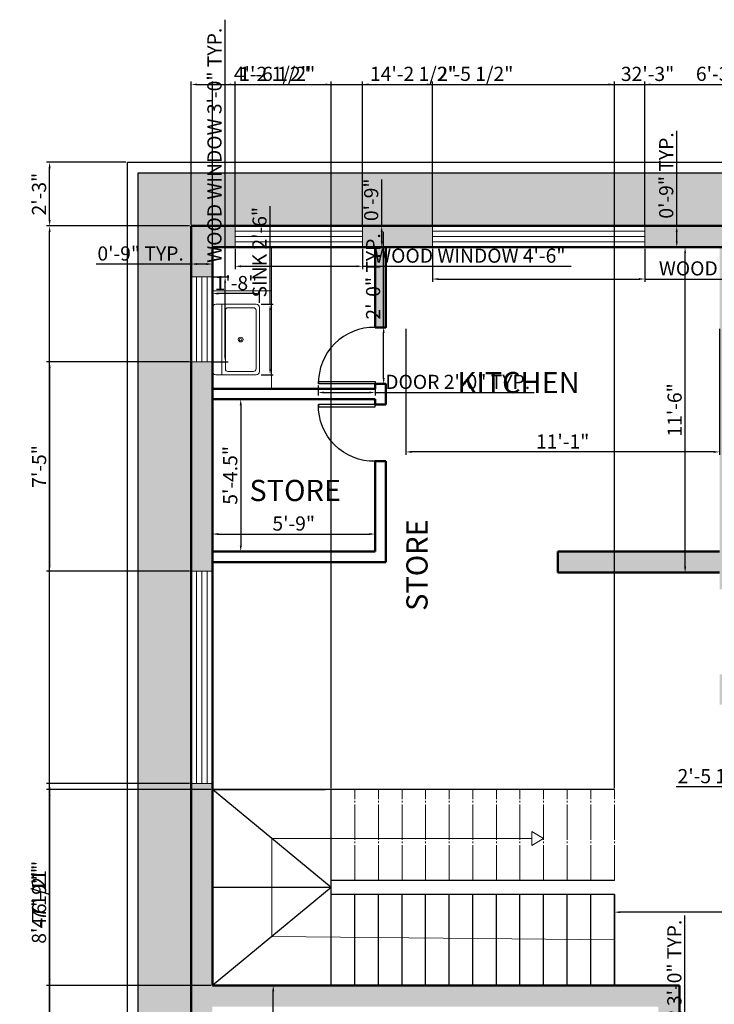
# Model space of a CAD drawing. Units: inches. Extents: x 2623 to 3157, y 1514 to 2273.
# Tile 4 of 6: x 2623 to 2917, y 1856 to 2273. Entities that reach past the tile are written whole.
import ezdxf

# ---------------------------------------------------------------- set-up
doc = ezdxf.new("R2010")
doc.units = ezdxf.units.IN
doc.linetypes.add('JIS_08_15', pattern=[17.25, 15, -0.75, 0.75, -0.75])
for name, color, linetype, lineweight in [('A-ANNO-DIMS', 2, 'Continuous', 18), ('A-ANNO-SYMB', 2, 'Continuous', 18), ('A-AREA-IDEN', 7, 'Continuous', 25), ('A-DOOR', 4, 'Continuous', 25), ('A-FLOR-CASE', 8, 'Continuous', 20), ('A-FLOR-FIXT', 9, 'Continuous', 18), ('A-FLOR-STRS', 7, 'Continuous', 25), ('A-FLOR-STRS-OVHD', 7, 'JIS_08_15', 18), ('A-GLAZ', 4, 'Continuous', 20), ('A-WALL', 7, 'Continuous', 50), ('A-WALL-PATT', 252, 'Continuous', 13), ('C-PROP', 7, 'Continuous', 25), ('L-PLNT-PATT', 9, 'Continuous', 13)]:
    doc.layers.add(name, color=color, linetype=linetype, lineweight=lineweight)
doc.styles.get("Standard").update_dxf_attribs({"font": 'arial.ttf'})
doc.dimstyles.new('ISO-25', dxfattribs={"dimtxt": 6, "dimasz": 2.5, "dimexe": 1.25, "dimexo": 0.625, "dimtad": 1, "dimdec": 1, "dimlunit": 3, "dimtxsty": 'Standard', "dimcen": 2.5, "dimadec": 0, "dimazin": 0, "dimtfac": 1, "dimtdec": 1, "dimtmove": 0, "dimatfit": 3, "dimfxl": 1, "dimarcsym": 0})

# ---------------------------------------------------------------- blocks, each defined once
blk = doc.blocks.new('Window - Wood Frame 36 in. Wide plan')
for p, q in [((0, 6), (0, 0)), ((36, 6), (36, 0)), ((0, 4.5), (36, 4.5)), ((0, 3), (36, 3)), ((0, 1.5), (36, 1.5))]:
    blk.add_line(p, q)
blk = doc.blocks.new('Sink-single - 30 in top')
blk.add_line((-15, -3.999996), (15, -3.999996))
for points in [[(-13.5, 0), (13.5, 0)], [(-15, -18.499996), (-15, -1.5)], [(15, -1.5), (15, -18.499996)], [(-13.5, -17.499996), (-13.5, -6.499996)], [(-12.5, -5.499996), (12.5, -5.499996)], [(13.5, -6.499996), (13.5, -17.499996)], [(13.5, -19.999996), (-13.5, -19.999996)], [(12.5, -18.499996), (-12.5, -18.499996)]]:
    blk.add_lwpolyline(points)
for radius in [1, 0.5]:
    blk.add_circle((0, -11.999996), radius)
for centre, radius, start, end in [((-13.5, -1.5), 1.5, 90, 180), ((13.5, -1.5), 1.5, 0, 90), ((-12.5, -6.499996), 1, 90, 180), ((12.5, -6.499996), 1, 0, 90), ((-13.5, -18.499996), 1.5, 180, 270), ((-12.5, -17.499996), 1, 180, 270), ((12.5, -17.499996), 1, 270, 0), ((13.5, -18.499996), 1.5, 270, 0)]:
    blk.add_arc(centre, radius, start, end)
blk = doc.blocks.new('*D12')
at = {"layer": 'A-ANNO-DIMS', "color": 0, "lineweight": -2, "transparency": 16777216}
for p, q in [((2704.92, 2112.15), (2717.58, 2112.15)), ((2716.33, 2109.65), (2716.33, 2050.15)), ((2704.92, 2047.65), (2717.58, 2047.65))]:
    blk.add_line(p, q, dxfattribs=at)
at = {"layer": 'A-ANNO-DIMS', "color": 0, "transparency": 16777216}
for points in [[(2715.91, 2109.65), (2716.75, 2109.65), (2716.33, 2112.15)], [(2715.91, 2050.15), (2716.75, 2050.15), (2716.33, 2047.65)]]:
    blk.add_solid(points, dxfattribs=at)
at = {"layer": 'Defpoints', "color": 0, "transparency": 16777216}
for p in [(2704.3, 2112.15), (2704.3, 2047.65), (2716.33, 2047.65)]:
    blk.add_point(p, dxfattribs=at)
at = {"layer": 'A-ANNO-DIMS', "color": 0, "transparency": 16777216, "insert": (2712.65, 2079.9), "char_height": 6, "attachment_point": 5, "rotation": 90}
blk.add_mtext('5\'-4.5"', dxfattribs=at)
blk = doc.blocks.new('*D13')
at = {"layer": 'A-ANNO-DIMS', "color": 0, "lineweight": -2, "transparency": 16777216}
for p, q in [((2704.3, 2048.27), (2704.3, 2056.27)), ((2706.8, 2055.02), (2770.8, 2055.02)), ((2773.3, 2048.27), (2773.3, 2056.27))]:
    blk.add_line(p, q, dxfattribs=at)
at = {"layer": 'A-ANNO-DIMS', "color": 0, "transparency": 16777216}
for points in [[(2706.8, 2055.44), (2706.8, 2054.6), (2704.3, 2055.02)], [(2770.8, 2055.44), (2770.8, 2054.6), (2773.3, 2055.02)]]:
    blk.add_solid(points, dxfattribs=at)
at = {"layer": 'Defpoints', "color": 0, "transparency": 16777216}
for p in [(2773.3, 2055.02), (2704.3, 2047.65), (2773.3, 2047.65)]:
    blk.add_point(p, dxfattribs=at)
at = {"layer": 'A-ANNO-DIMS', "color": 0, "transparency": 16777216, "insert": (2738.8, 2058.71), "char_height": 6, "attachment_point": 5}
blk.add_mtext('5\'-9"', dxfattribs=at)
blk = doc.blocks.new('*D14')
at = {"layer": 'A-ANNO-DIMS', "color": 0, "lineweight": -2, "transparency": 16777216}
for p, q in [((2851.42, 2176.65), (2905.96, 2176.65)), ((2904.71, 2041.15), (2904.71, 2174.15)), ((2851.42, 2038.65), (2905.96, 2038.65))]:
    blk.add_line(p, q, dxfattribs=at)
at = {"layer": 'A-ANNO-DIMS', "color": 0, "transparency": 16777216}
for points in [[(2904.3, 2174.15), (2905.13, 2174.15), (2904.71, 2176.65)], [(2904.3, 2041.15), (2905.13, 2041.15), (2904.71, 2038.65)]]:
    blk.add_solid(points, dxfattribs=at)
at = {"layer": 'Defpoints', "color": 0, "transparency": 16777216}
for p in [(2850.8, 2176.65), (2904.71, 2176.65), (2850.8, 2038.65)]:
    blk.add_point(p, dxfattribs=at)
at = {"layer": 'A-ANNO-DIMS', "color": 0, "transparency": 16777216, "insert": (2901.03, 2107.65), "char_height": 6, "attachment_point": 5, "rotation": 90}
blk.add_mtext('11\'-6"', dxfattribs=at)
blk = doc.blocks.new('*D15')
at = {"layer": 'A-ANNO-DIMS', "color": 0, "lineweight": -2, "transparency": 16777216}
for p, q in [((2786.3, 2142.02), (2786.3, 2088.59)), ((2919.3, 2142.02), (2919.3, 2088.59)), ((2916.8, 2089.84), (2788.8, 2089.84))]:
    blk.add_line(p, q, dxfattribs=at)
at = {"layer": 'A-ANNO-DIMS', "color": 0, "transparency": 16777216}
for points in [[(2788.8, 2090.25), (2788.8, 2089.42), (2786.3, 2089.84)], [(2916.8, 2090.25), (2916.8, 2089.42), (2919.3, 2089.84)]]:
    blk.add_solid(points, dxfattribs=at)
at = {"layer": 'Defpoints', "color": 0, "transparency": 16777216}
for p in [(2786.3, 2142.65), (2919.3, 2142.65), (2786.3, 2089.84)]:
    blk.add_point(p, dxfattribs=at)
at = {"layer": 'A-ANNO-DIMS', "color": 0, "transparency": 16777216, "insert": (2852.8, 2093.47), "char_height": 6, "attachment_point": 5}
blk.add_mtext('11\'-1"', dxfattribs=at)
blk = doc.blocks.new('*D22')
at = {"layer": 'A-ANNO-DIMS', "color": 0, "lineweight": -2, "transparency": 16777216}
for p, q in [((2874.71, 1864.27), (2874.71, 1895.95)), ((3082.3, 1857.21), (3082.3, 1895.95)), ((3079.8, 1894.7), (2877.21, 1894.7))]:
    blk.add_line(p, q, dxfattribs=at)
at = {"layer": 'A-ANNO-DIMS', "color": 0, "transparency": 16777216}
for points in [[(2877.21, 1895.12), (2877.21, 1894.28), (2874.71, 1894.7)], [(3079.8, 1895.12), (3079.8, 1894.28), (3082.3, 1894.7)]]:
    blk.add_solid(points, dxfattribs=at)
at = {"layer": 'Defpoints', "color": 0, "transparency": 16777216}
for p in [(2874.71, 1894.7), (2874.71, 1863.65), (3082.3, 1856.59)]:
    blk.add_point(p, dxfattribs=at)
at = {"layer": 'A-ANNO-DIMS', "color": 0, "transparency": 16777216, "insert": (2978.5, 1898.39), "char_height": 6, "attachment_point": 5}
blk.add_mtext('17\'-3.6"', dxfattribs=at)
blk = doc.blocks.new('*D27')
at = {"layer": 'A-ANNO-DIMS', "color": 0, "lineweight": -2, "transparency": 16777216}
for p, q in [((2704.92, 1863.65), (2731.35, 1863.65)), ((2730.1, 1810.15), (2730.1, 1861.15)), ((2704.92, 1807.65), (2731.35, 1807.65))]:
    blk.add_line(p, q, dxfattribs=at)
at = {"layer": 'A-ANNO-DIMS', "color": 0, "transparency": 16777216}
for points in [[(2729.68, 1861.15), (2730.51, 1861.15), (2730.1, 1863.65)], [(2729.68, 1810.15), (2730.51, 1810.15), (2730.1, 1807.65)]]:
    blk.add_solid(points, dxfattribs=at)
at = {"layer": 'Defpoints', "color": 0, "transparency": 16777216}
for p in [(2704.3, 1863.65), (2730.1, 1863.65), (2704.3, 1807.65)]:
    blk.add_point(p, dxfattribs=at)
at = {"layer": 'A-ANNO-DIMS', "color": 0, "transparency": 16777216, "insert": (2726.41, 1835.65), "char_height": 6, "attachment_point": 5, "rotation": 90}
blk.add_mtext('4\'-8"', dxfattribs=at)
blk = doc.blocks.new('DOOR-SWING-24IN')
for p, q in [((0, 0), (0, 1)), ((0, 1), (24, 1)), ((24, 0), (0, 0)), ((24, 1), (24, 0))]:
    blk.add_line(p, q)
blk.add_arc((23.5, 0.5), 23.51, 88.7811, 181.2189)
blk = doc.blocks.new('*D31')
at = {"layer": 'A-ANNO-DIMS', "color": 0, "lineweight": -2, "transparency": 16777216}
for p, q in [((2797.66, 2176.02), (2797.66, 2161.9)), ((2887.66, 2176.02), (2887.66, 2161.9)), ((2800.16, 2163.15), (2885.16, 2163.15)), ((2887.66, 2163.15), (2996.67, 2163.15))]:
    blk.add_line(p, q, dxfattribs=at)
at = {"layer": 'A-ANNO-DIMS', "color": 0, "transparency": 16777216}
for points in [[(2800.16, 2163.56), (2800.16, 2162.73), (2797.66, 2163.15)], [(2885.16, 2163.56), (2885.16, 2162.73), (2887.66, 2163.15)]]:
    blk.add_solid(points, dxfattribs=at)
at = {"layer": 'Defpoints', "color": 0, "transparency": 16777216}
for p in [(2797.66, 2176.65), (2887.66, 2176.65), (2887.66, 2163.15)]:
    blk.add_point(p, dxfattribs=at)
at = {"layer": 'A-ANNO-DIMS', "color": 0, "transparency": 16777216, "insert": (2943.42, 2166.88), "char_height": 6, "attachment_point": 5}
blk.add_mtext('WOOD WINDOW 7\'-6" TYP.', dxfattribs=at)
blk = doc.blocks.new('*D32')
at = {"layer": 'A-ANNO-DIMS', "color": 0, "lineweight": -2, "transparency": 16777216}
for p, q in [((2901.16, 2185.65), (2901.16, 2225.97)), ((2888.29, 2185.65), (2902.41, 2185.65)), ((2901.16, 2179.15), (2901.16, 2183.15)), ((2888.29, 2176.65), (2902.41, 2176.65))]:
    blk.add_line(p, q, dxfattribs=at)
at = {"layer": 'A-ANNO-DIMS', "color": 0, "transparency": 16777216}
for points in [[(2900.75, 2183.15), (2901.58, 2183.15), (2901.16, 2185.65)], [(2900.75, 2179.15), (2901.58, 2179.15), (2901.16, 2176.65)]]:
    blk.add_solid(points, dxfattribs=at)
at = {"layer": 'Defpoints', "color": 0, "transparency": 16777216}
for p in [(2887.66, 2185.65), (2901.16, 2185.65), (2887.66, 2176.65)]:
    blk.add_point(p, dxfattribs=at)
at = {"layer": 'A-ANNO-DIMS', "color": 0, "transparency": 16777216, "insert": (2897.48, 2207.06), "char_height": 6, "attachment_point": 5, "rotation": 90}
blk.add_mtext('0\'-9" TYP.', dxfattribs=at)
blk = doc.blocks.new('*D33')
at = {"layer": 'A-ANNO-DIMS', "color": 0, "lineweight": -2, "transparency": 16777216}
for p, q in [((2714, 2176.02), (2714, 2167.3)), ((2768, 2176.02), (2768, 2167.3)), ((2716.5, 2168.55), (2765.5, 2168.55)), ((2768, 2168.55), (2856.39, 2168.55))]:
    blk.add_line(p, q, dxfattribs=at)
at = {"layer": 'A-ANNO-DIMS', "color": 0, "transparency": 16777216}
for points in [[(2716.5, 2168.96), (2716.5, 2168.13), (2714, 2168.55)], [(2765.5, 2168.96), (2765.5, 2168.13), (2768, 2168.55)]]:
    blk.add_solid(points, dxfattribs=at)
at = {"layer": 'Defpoints', "color": 0, "transparency": 16777216}
for p in [(2714, 2176.65), (2768, 2176.65), (2768, 2168.55)]:
    blk.add_point(p, dxfattribs=at)
at = {"layer": 'A-ANNO-DIMS', "color": 0, "transparency": 16777216, "insert": (2813.45, 2172.28), "char_height": 6, "attachment_point": 5}
blk.add_mtext('WOOD WINDOW 4\'-6"', dxfattribs=at)
blk = doc.blocks.new('*D34')
at = {"layer": 'A-ANNO-DIMS', "color": 0, "lineweight": -2, "transparency": 16777216}
for p, q in [((2776.1, 2185.65), (2776.1, 2205.35)), ((2768.63, 2185.65), (2777.35, 2185.65)), ((2776.1, 2179.15), (2776.1, 2183.15)), ((2768.63, 2176.65), (2777.35, 2176.65))]:
    blk.add_line(p, q, dxfattribs=at)
at = {"layer": 'A-ANNO-DIMS', "color": 0, "transparency": 16777216}
for points in [[(2775.69, 2183.15), (2776.52, 2183.15), (2776.1, 2185.65)], [(2775.69, 2179.15), (2776.52, 2179.15), (2776.1, 2176.65)]]:
    blk.add_solid(points, dxfattribs=at)
at = {"layer": 'Defpoints', "color": 0, "transparency": 16777216}
for p in [(2768, 2185.65), (2776.1, 2185.65), (2768, 2176.65)]:
    blk.add_point(p, dxfattribs=at)
at = {"layer": 'A-ANNO-DIMS', "color": 0, "transparency": 16777216, "insert": (2772.41, 2196.75), "char_height": 6, "attachment_point": 5, "rotation": 90}
blk.add_mtext('0\'-9"', dxfattribs=at)
blk = doc.blocks.new('*D35')
at = {"layer": 'A-ANNO-DIMS', "color": 0, "lineweight": -2, "transparency": 16777216}
for p, q in [((2709.7, 2164.1), (2709.7, 2273.11)), ((2704.92, 2164.1), (2710.95, 2164.1)), ((2709.7, 2130.6), (2709.7, 2161.6)), ((2704.92, 2128.1), (2710.95, 2128.1))]:
    blk.add_line(p, q, dxfattribs=at)
at = {"layer": 'A-ANNO-DIMS', "color": 0, "transparency": 16777216}
for points in [[(2709.28, 2161.6), (2710.11, 2161.6), (2709.7, 2164.1)], [(2709.28, 2130.6), (2710.11, 2130.6), (2709.7, 2128.1)]]:
    blk.add_solid(points, dxfattribs=at)
at = {"layer": 'Defpoints', "color": 0, "transparency": 16777216}
for p in [(2704.3, 2164.1), (2709.7, 2164.1), (2704.3, 2128.1)]:
    blk.add_point(p, dxfattribs=at)
at = {"layer": 'A-ANNO-DIMS', "color": 0, "transparency": 16777216, "insert": (2705.96, 2219.86), "char_height": 6, "attachment_point": 5, "rotation": 90}
blk.add_mtext('WOOD WINDOW 3\'-0" TYP.', dxfattribs=at)
blk = doc.blocks.new('*D36')
at = {"layer": 'A-ANNO-DIMS', "color": 0, "lineweight": -2, "transparency": 16777216}
for p, q in [((2695.3, 2169.5), (2654.97, 2169.5)), ((2695.3, 2164.73), (2695.3, 2170.75)), ((2701.8, 2169.5), (2697.8, 2169.5)), ((2704.3, 2164.73), (2704.3, 2170.75))]:
    blk.add_line(p, q, dxfattribs=at)
at = {"layer": 'A-ANNO-DIMS', "color": 0, "transparency": 16777216}
for points in [[(2697.8, 2169.92), (2697.8, 2169.09), (2695.3, 2169.5)], [(2701.8, 2169.92), (2701.8, 2169.09), (2704.3, 2169.5)]]:
    blk.add_solid(points, dxfattribs=at)
at = {"layer": 'Defpoints', "color": 0, "transparency": 16777216}
for p in [(2695.3, 2169.5), (2695.3, 2164.1), (2704.3, 2164.1)]:
    blk.add_point(p, dxfattribs=at)
at = {"layer": 'A-ANNO-DIMS', "color": 0, "transparency": 16777216, "insert": (2673.88, 2173.19), "char_height": 6, "attachment_point": 5}
blk.add_mtext('0\'-9" TYP.', dxfattribs=at)
blk = doc.blocks.new('*D37')
at = {"layer": 'A-ANNO-DIMS', "color": 0, "lineweight": -2, "transparency": 16777216}
for p, q in [((2749.16, 2118.02), (2749.16, 2113.78)), ((2773.3, 2118.02), (2773.3, 2113.78)), ((2751.66, 2115.03), (2770.8, 2115.03)), ((2773.3, 2115.03), (2840.79, 2115.03))]:
    blk.add_line(p, q, dxfattribs=at)
at = {"layer": 'A-ANNO-DIMS', "color": 0, "transparency": 16777216}
for points in [[(2751.66, 2115.44), (2751.66, 2114.61), (2749.16, 2115.03)], [(2770.8, 2115.44), (2770.8, 2114.61), (2773.3, 2115.03)]]:
    blk.add_solid(points, dxfattribs=at)
at = {"layer": 'Defpoints', "color": 0, "transparency": 16777216}
for p in [(2749.16, 2118.65), (2773.3, 2118.65), (2773.3, 2115.03)]:
    blk.add_point(p, dxfattribs=at)
at = {"layer": 'A-ANNO-DIMS', "color": 0, "transparency": 16777216, "insert": (2808.3, 2118.76), "char_height": 6, "attachment_point": 5}
blk.add_mtext('DOOR 2\'-0" TYP.', dxfattribs=at)
blk = doc.blocks.new('*D38')
at = {"layer": 'A-ANNO-DIMS', "color": 0, "lineweight": -2, "transparency": 16777216}
for p, q in [((2776.92, 2142.78), (2776.92, 2183.21)), ((2773.92, 2142.78), (2778.17, 2142.78)), ((2776.92, 2121.15), (2776.92, 2140.28)), ((2773.92, 2118.65), (2778.17, 2118.65))]:
    blk.add_line(p, q, dxfattribs=at)
at = {"layer": 'A-ANNO-DIMS', "color": 0, "transparency": 16777216}
for points in [[(2776.5, 2140.28), (2777.33, 2140.28), (2776.92, 2142.78)], [(2776.5, 2121.15), (2777.33, 2121.15), (2776.92, 2118.65)]]:
    blk.add_solid(points, dxfattribs=at)
at = {"layer": 'Defpoints', "color": 0, "transparency": 16777216}
for p in [(2773.3, 2142.78), (2776.92, 2142.78), (2773.3, 2118.65)]:
    blk.add_point(p, dxfattribs=at)
at = {"layer": 'A-ANNO-DIMS', "color": 0, "transparency": 16777216, "insert": (2773.23, 2164.25), "char_height": 6, "attachment_point": 5, "rotation": 90}
blk.add_mtext('2\'-0" TYP.', dxfattribs=at)
blk = doc.blocks.new('*D39')
at = {"layer": 'A-ANNO-DIMS', "color": 0, "lineweight": -2, "transparency": 16777216}
for p, q in [((2904.66, 1825.78), (2904.66, 1893.28)), ((2909.45, 1825.78), (2903.41, 1825.78)), ((2904.66, 1792.15), (2904.66, 1823.28)), ((2909.45, 1789.65), (2903.41, 1789.65))]:
    blk.add_line(p, q, dxfattribs=at)
at = {"layer": 'A-ANNO-DIMS', "color": 0, "transparency": 16777216}
for points in [[(2904.24, 1823.28), (2905.08, 1823.28), (2904.66, 1825.78)], [(2904.24, 1792.15), (2905.08, 1792.15), (2904.66, 1789.65)]]:
    blk.add_solid(points, dxfattribs=at)
at = {"layer": 'Defpoints', "color": 0, "transparency": 16777216}
for p in [(2904.66, 1825.78), (2910.08, 1825.78), (2910.08, 1789.65)]:
    blk.add_point(p, dxfattribs=at)
at = {"layer": 'A-ANNO-DIMS', "color": 0, "transparency": 16777216, "insert": (2900.93, 1860.78), "char_height": 6, "attachment_point": 5, "rotation": 90}
blk.add_mtext('DOOR 3\'-0" TYP.', dxfattribs=at)
blk = doc.blocks.new('*D46')
at = {"layer": 'A-ANNO-DIMS', "color": 0, "lineweight": -2, "transparency": 16777216}
for p, q in [((2955.35, 1947.87), (2900.94, 1947.87)), ((2955.35, 1941.29), (2955.35, 1949.12)), ((2982.18, 1947.87), (2957.85, 1947.87)), ((2984.68, 1941.29), (2984.68, 1949.12))]:
    blk.add_line(p, q, dxfattribs=at)
at = {"layer": 'A-ANNO-DIMS', "color": 0, "transparency": 16777216}
for points in [[(2957.85, 1948.29), (2957.85, 1947.45), (2955.35, 1947.87)], [(2982.18, 1948.29), (2982.18, 1947.45), (2984.68, 1947.87)]]:
    blk.add_solid(points, dxfattribs=at)
at = {"layer": 'Defpoints', "color": 0, "transparency": 16777216}
for p in [(2955.35, 1947.87), (2955.35, 1940.67), (2984.68, 1940.67)]:
    blk.add_point(p, dxfattribs=at)
at = {"layer": 'A-ANNO-DIMS', "color": 0, "transparency": 16777216, "insert": (2926.89, 1951.6), "char_height": 6, "attachment_point": 5}
blk.add_mtext('2\'-5 1/2" TYP.', dxfattribs=at)
blk = doc.blocks.new('*D55')
at = {"layer": 'A-ANNO-DIMS', "color": 0, "lineweight": -2, "transparency": 16777216}
for p, q in [((2728.8, 2152.49), (2728.8, 2194.05)), ((2724.92, 2152.49), (2730.05, 2152.49)), ((2728.8, 2124.99), (2728.8, 2149.99)), ((2724.92, 2122.49), (2730.05, 2122.49))]:
    blk.add_line(p, q, dxfattribs=at)
at = {"layer": 'A-ANNO-DIMS', "color": 0, "transparency": 16777216}
for points in [[(2728.38, 2149.99), (2729.21, 2149.99), (2728.8, 2152.49)], [(2728.38, 2124.99), (2729.21, 2124.99), (2728.8, 2122.49)]]:
    blk.add_solid(points, dxfattribs=at)
at = {"layer": 'Defpoints', "color": 0, "transparency": 16777216}
for p in [(2724.3, 2152.49), (2728.8, 2152.49), (2724.3, 2122.49)]:
    blk.add_point(p, dxfattribs=at)
at = {"layer": 'A-ANNO-DIMS', "color": 0, "transparency": 16777216, "insert": (2725.07, 2174.52), "char_height": 6, "attachment_point": 5, "rotation": 90}
blk.add_mtext('SINK 2\'-6"', dxfattribs=at)
blk = doc.blocks.new('*D56')
at = {"layer": 'A-ANNO-DIMS', "color": 0, "lineweight": -2, "transparency": 16777216}
for p, q in [((2704.3, 2153.11), (2704.3, 2158.24)), ((2721.8, 2156.99), (2706.8, 2156.99)), ((2724.3, 2153.11), (2724.3, 2158.24))]:
    blk.add_line(p, q, dxfattribs=at)
at = {"layer": 'A-ANNO-DIMS', "color": 0, "transparency": 16777216}
for points in [[(2706.8, 2157.4), (2706.8, 2156.57), (2704.3, 2156.99)], [(2721.8, 2157.4), (2721.8, 2156.57), (2724.3, 2156.99)]]:
    blk.add_solid(points, dxfattribs=at)
at = {"layer": 'Defpoints', "color": 0, "transparency": 16777216}
for p in [(2704.3, 2156.99), (2704.3, 2152.49), (2724.3, 2152.49)]:
    blk.add_point(p, dxfattribs=at)
at = {"layer": 'A-ANNO-DIMS', "color": 0, "transparency": 16777216, "insert": (2714.3, 2160.67), "char_height": 6, "attachment_point": 5}
blk.add_mtext('1\'-8"', dxfattribs=at)
blk = doc.blocks.new('*D61')
at = {"layer": 'A-ANNO-DIMS', "color": 0, "lineweight": -2, "transparency": 16777216}
for p, q in [((2695.3, 2186.27), (2695.3, 2246.9)), ((3082.3, 2186.27), (3082.3, 2246.9)), ((2697.8, 2245.65), (3079.8, 2245.65))]:
    blk.add_line(p, q, dxfattribs=at)
at = {"layer": 'A-ANNO-DIMS', "color": 0, "transparency": 16777216}
for points in [[(2697.8, 2246.06), (2697.8, 2245.23), (2695.3, 2245.65)], [(3079.8, 2246.06), (3079.8, 2245.23), (3082.3, 2245.65)]]:
    blk.add_solid(points, dxfattribs=at)
at = {"layer": 'Defpoints', "color": 0, "transparency": 16777216}
for p in [(3082.3, 2245.65), (2695.3, 2185.65), (3082.3, 2185.65)]:
    blk.add_point(p, dxfattribs=at)
at = {"layer": 'A-ANNO-DIMS', "color": 0, "transparency": 16777216, "insert": (2888.8, 2249.34), "char_height": 6, "attachment_point": 5}
blk.add_mtext('32\'-3"', dxfattribs=at)
blk = doc.blocks.new('*D62')
at = {"layer": 'A-ANNO-DIMS', "color": 0, "lineweight": -2, "transparency": 16777216}
for p, q in [((2694.67, 2185.65), (2634.05, 2185.65)), ((2635.3, 1615.15), (2635.3, 2183.15)), ((2694.67, 1612.65), (2634.05, 1612.65))]:
    blk.add_line(p, q, dxfattribs=at)
at = {"layer": 'A-ANNO-DIMS', "color": 0, "transparency": 16777216}
for points in [[(2634.88, 2183.15), (2635.71, 2183.15), (2635.3, 2185.65)], [(2634.88, 1615.15), (2635.71, 1615.15), (2635.3, 1612.65)]]:
    blk.add_solid(points, dxfattribs=at)
at = {"layer": 'Defpoints', "color": 0, "transparency": 16777216}
for p in [(2635.3, 2185.65), (2695.3, 2185.65), (2695.3, 1612.65)]:
    blk.add_point(p, dxfattribs=at)
at = {"layer": 'A-ANNO-DIMS', "color": 0, "transparency": 16777216, "insert": (2631.61, 1899.15), "char_height": 6, "attachment_point": 5, "rotation": 90}
blk.add_mtext('47\'-9"', dxfattribs=at)
blk = doc.blocks.new('*D64')
at = {"layer": 'A-ANNO-DIMS', "color": 0, "lineweight": -2, "transparency": 16777216}
for p, q in [((2667.67, 2212.65), (2634.05, 2212.65)), ((2635.3, 2188.15), (2635.3, 2210.15)), ((2694.67, 2185.65), (2634.05, 2185.65))]:
    blk.add_line(p, q, dxfattribs=at)
at = {"layer": 'A-ANNO-DIMS', "color": 0, "transparency": 16777216}
for points in [[(2634.88, 2210.15), (2635.71, 2210.15), (2635.3, 2212.65)], [(2634.88, 2188.15), (2635.71, 2188.15), (2635.3, 2185.65)]]:
    blk.add_solid(points, dxfattribs=at)
at = {"layer": 'Defpoints', "color": 0, "transparency": 16777216}
for p in [(2635.3, 2212.65), (2668.3, 2212.65), (2695.3, 2185.65)]:
    blk.add_point(p, dxfattribs=at)
at = {"layer": 'A-ANNO-DIMS', "color": 0, "transparency": 16777216, "insert": (2631.6, 2199.15), "char_height": 6, "attachment_point": 5, "rotation": 90}
blk.add_mtext('2\'-3"', dxfattribs=at)
blk = doc.blocks.new('*D69')
at = {"layer": 'A-ANNO-DIMS', "color": 0, "lineweight": -2, "transparency": 16777216}
for p, q in [((2704.3, 1947.27), (2704.3, 2246.9)), ((2874.71, 1947.27), (2874.71, 2246.9)), ((2706.8, 2245.65), (2872.21, 2245.65))]:
    blk.add_line(p, q, dxfattribs=at)
at = {"layer": 'A-ANNO-DIMS', "color": 0, "transparency": 16777216}
for points in [[(2706.8, 2246.06), (2706.8, 2245.23), (2704.3, 2245.65)], [(2872.21, 2246.06), (2872.21, 2245.23), (2874.71, 2245.65)]]:
    blk.add_solid(points, dxfattribs=at)
at = {"layer": 'Defpoints', "color": 0, "transparency": 16777216}
for p in [(2874.71, 2245.65), (2704.3, 1946.65), (2874.71, 1946.65)]:
    blk.add_point(p, dxfattribs=at)
at = {"layer": 'A-ANNO-DIMS', "color": 0, "transparency": 16777216, "insert": (2789.5, 2249.37), "char_height": 6, "attachment_point": 5}
blk.add_mtext('14\'-2 1/2"', dxfattribs=at)
blk = doc.blocks.new('*D70')
at = {"layer": 'A-ANNO-DIMS', "color": 0, "lineweight": -2, "transparency": 16777216}
for p, q in [((2703.67, 1946.65), (2634.05, 1946.65)), ((2635.3, 1866.15), (2635.3, 1944.15)), ((2703.67, 1863.65), (2634.05, 1863.65))]:
    blk.add_line(p, q, dxfattribs=at)
at = {"layer": 'A-ANNO-DIMS', "color": 0, "transparency": 16777216}
for points in [[(2634.88, 1944.15), (2635.71, 1944.15), (2635.3, 1946.65)], [(2634.88, 1866.15), (2635.71, 1866.15), (2635.3, 1863.65)]]:
    blk.add_solid(points, dxfattribs=at)
at = {"layer": 'Defpoints', "color": 0, "transparency": 16777216}
for p in [(2635.3, 1946.65), (2704.3, 1946.65), (2704.3, 1863.65)]:
    blk.add_point(p, dxfattribs=at)
at = {"layer": 'A-ANNO-DIMS', "color": 0, "transparency": 16777216, "insert": (2631.61, 1905.15), "char_height": 6, "attachment_point": 5, "rotation": 90}
blk.add_mtext('6\'-11"', dxfattribs=at)
blk = doc.blocks.new('*D76')
at = {"layer": 'A-ANNO-DIMS', "color": 0, "lineweight": -2, "transparency": 16777216}
for p, q in [((2695.3, 2186.27), (2695.3, 2246.9)), ((2714, 2186.27), (2714, 2246.9)), ((2697.8, 2245.65), (2711.5, 2245.65)), ((2714, 2245.65), (2747.12, 2245.65))]:
    blk.add_line(p, q, dxfattribs=at)
at = {"layer": 'A-ANNO-DIMS', "color": 0, "transparency": 16777216}
for points in [[(2697.8, 2246.06), (2697.8, 2245.23), (2695.3, 2245.65)], [(2711.5, 2246.06), (2711.5, 2245.23), (2714, 2245.65)]]:
    blk.add_solid(points, dxfattribs=at)
at = {"layer": 'Defpoints', "color": 0, "transparency": 16777216}
for p in [(2714, 2245.65), (2695.3, 2185.65), (2714, 2185.65)]:
    blk.add_point(p, dxfattribs=at)
at = {"layer": 'A-ANNO-DIMS', "color": 0, "transparency": 16777216, "insert": (2731.81, 2249.37), "char_height": 6, "attachment_point": 5}
blk.add_mtext('1\'-6 1/2"', dxfattribs=at)
blk = doc.blocks.new('*D77')
at = {"layer": 'A-ANNO-DIMS', "color": 0, "lineweight": -2, "transparency": 16777216}
for p, q in [((2768, 2186.27), (2768, 2246.9)), ((2797.66, 2186.27), (2797.66, 2246.9)), ((2770.5, 2245.65), (2795.16, 2245.65)), ((2797.66, 2245.65), (2831.45, 2245.65))]:
    blk.add_line(p, q, dxfattribs=at)
at = {"layer": 'A-ANNO-DIMS', "color": 0, "transparency": 16777216}
for points in [[(2770.5, 2246.06), (2770.5, 2245.23), (2768, 2245.65)], [(2795.16, 2246.06), (2795.16, 2245.23), (2797.66, 2245.65)]]:
    blk.add_solid(points, dxfattribs=at)
at = {"layer": 'Defpoints', "color": 0, "transparency": 16777216}
for p in [(2797.66, 2245.65), (2768, 2185.65), (2797.66, 2185.65)]:
    blk.add_point(p, dxfattribs=at)
at = {"layer": 'A-ANNO-DIMS', "color": 0, "transparency": 16777216, "insert": (2815.8, 2249.37), "char_height": 6, "attachment_point": 5}
blk.add_mtext('2\'-5 1/2"', dxfattribs=at)
blk = doc.blocks.new('*D78')
at = {"layer": 'A-ANNO-DIMS', "color": 0, "lineweight": -2, "transparency": 16777216}
for p, q in [((2887.66, 2186.27), (2887.66, 2246.9)), ((2963.13, 2186.27), (2963.13, 2246.9)), ((2890.16, 2245.65), (2960.63, 2245.65))]:
    blk.add_line(p, q, dxfattribs=at)
at = {"layer": 'A-ANNO-DIMS', "color": 0, "transparency": 16777216}
for points in [[(2890.16, 2246.06), (2890.16, 2245.23), (2887.66, 2245.65)], [(2960.63, 2246.06), (2960.63, 2245.23), (2963.13, 2245.65)]]:
    blk.add_solid(points, dxfattribs=at)
at = {"layer": 'Defpoints', "color": 0, "transparency": 16777216}
for p in [(2963.13, 2245.65), (2887.66, 2185.65), (2963.13, 2185.65)]:
    blk.add_point(p, dxfattribs=at)
at = {"layer": 'A-ANNO-DIMS', "color": 0, "transparency": 16777216, "insert": (2925.4, 2249.38), "char_height": 6, "attachment_point": 5}
blk.add_mtext('6\'-3 1/2"', dxfattribs=at)
blk = doc.blocks.new('*D85')
at = {"layer": 'A-ANNO-DIMS', "color": 0, "lineweight": -2, "transparency": 16777216}
for p, q in [((2704.3, 1947.27), (2704.3, 2246.9)), ((2754.71, 1947.27), (2754.71, 2246.9)), ((2706.8, 2245.65), (2752.21, 2245.65))]:
    blk.add_line(p, q, dxfattribs=at)
at = {"layer": 'A-ANNO-DIMS', "color": 0, "transparency": 16777216}
for points in [[(2706.8, 2246.06), (2706.8, 2245.23), (2704.3, 2245.65)], [(2752.21, 2246.06), (2752.21, 2245.23), (2754.71, 2245.65)]]:
    blk.add_solid(points, dxfattribs=at)
at = {"layer": 'Defpoints', "color": 0, "transparency": 16777216}
for p in [(2754.71, 2245.65), (2704.3, 1946.65), (2754.71, 1946.65)]:
    blk.add_point(p, dxfattribs=at)
at = {"layer": 'A-ANNO-DIMS', "color": 0, "transparency": 16777216, "insert": (2729.5, 2249.37), "char_height": 6, "attachment_point": 5}
blk.add_mtext('4\'-2 1/2"', dxfattribs=at)
blk = doc.blocks.new('*D89')
at = {"layer": 'A-ANNO-DIMS', "color": 0, "lineweight": -2, "transparency": 16777216}
for p, q in [((2694.67, 2128.1), (2634.05, 2128.1)), ((2635.3, 2125.6), (2635.3, 2041.75)), ((2694.67, 2039.25), (2634.05, 2039.25))]:
    blk.add_line(p, q, dxfattribs=at)
at = {"layer": 'A-ANNO-DIMS', "color": 0, "transparency": 16777216}
for points in [[(2634.88, 2125.6), (2635.71, 2125.6), (2635.3, 2128.1)], [(2634.88, 2041.75), (2635.71, 2041.75), (2635.3, 2039.25)]]:
    blk.add_solid(points, dxfattribs=at)
at = {"layer": 'Defpoints', "color": 0, "transparency": 16777216}
for p in [(2695.3, 2128.1), (2635.3, 2039.25), (2695.3, 2039.25)]:
    blk.add_point(p, dxfattribs=at)
at = {"layer": 'A-ANNO-DIMS', "color": 0, "transparency": 16777216, "insert": (2631.62, 2083.68), "char_height": 6, "attachment_point": 5, "rotation": 90}
blk.add_mtext('7\'-5"', dxfattribs=at)
blk = doc.blocks.new('*D90')
at = {"layer": 'A-ANNO-DIMS', "color": 0, "lineweight": -2, "transparency": 16777216}
for p, q in [((2694.67, 1949.25), (2634.05, 1949.25)), ((2635.3, 1946.75), (2635.3, 1848.07)), ((2694.67, 1845.57), (2634.05, 1845.57))]:
    blk.add_line(p, q, dxfattribs=at)
at = {"layer": 'A-ANNO-DIMS', "color": 0, "transparency": 16777216}
for points in [[(2634.88, 1946.75), (2635.71, 1946.75), (2635.3, 1949.25)], [(2634.88, 1848.07), (2635.71, 1848.07), (2635.3, 1845.57)]]:
    blk.add_solid(points, dxfattribs=at)
at = {"layer": 'Defpoints', "color": 0, "transparency": 16777216}
for p in [(2695.3, 1949.25), (2635.3, 1845.57), (2695.3, 1845.57)]:
    blk.add_point(p, dxfattribs=at)
at = {"layer": 'A-ANNO-DIMS', "color": 0, "transparency": 16777216, "insert": (2631.57, 1897.41), "char_height": 6, "attachment_point": 5, "rotation": 90}
blk.add_mtext('8\'-7 1/2"', dxfattribs=at)

msp = doc.modelspace()

# ---------------------------------------------------------------- hatches: boundary and pattern name
at = {"layer": 'A-WALL-PATT'}
h = msp.add_hatch(color=256, dxfattribs=at)
h.dxf.hatch_style = 1
h.paths.add_polyline_path([(2704.3, 1854.65), (2893.38, 1854.65), (2893.38, 1850.02), (2902.38, 1850.02), (2902.38, 1863.65), (2704.3, 1863.65), (2704.3, 1949.25), (2695.3, 1949.25), (2695.3, 1845.57), (2704.3, 1845.57)])
h.paths.add_polyline_path([(2704.3, 1809.57), (2695.3, 1809.57), (2695.3, 1750.74), (2704.3, 1750.74)])
h.paths.add_polyline_path([(2764.7, 1621.65), (2704.3, 1621.65), (2704.3, 1660.74), (2695.3, 1660.74), (2695.3, 1612.65), (2764.7, 1612.65)])
h.paths.add_polyline_path([(2704.3, 2128.1), (2695.3, 2128.1), (2695.3, 2039.25), (2704.3, 2039.25)])
h.paths.add_polyline_path([(2714, 2185.65), (2695.3, 2185.65), (2695.3, 2164.1), (2704.3, 2164.1), (2704.3, 2176.65), (2714, 2176.65)])
h.paths.add_polyline_path([(2797.66, 2185.65), (2768, 2185.65), (2768, 2176.65), (2797.66, 2176.65)])
h.paths.add_polyline_path([(2777.8, 2176.65), (2773.3, 2176.65), (2773.3, 2142.65), (2777.8, 2142.65)])
h.paths.add_polyline_path([(2963.13, 2185.65), (2887.66, 2185.65), (2887.66, 2176.65), (2963.13, 2176.65)])
h.paths.add_polyline_path([(2928.3, 2176.65), (2919.3, 2176.65), (2919.3, 2047.65), (2850.8, 2047.65), (2850.8, 2038.65), (2919.3, 2038.65), (2919.3, 2031.57), (2928.3, 2031.57), (2928.3, 2038.65)])
h.paths.add_polyline_path([(3082.3, 2185.65), (3053.13, 2185.65), (3053.13, 2176.65), (3073.3, 2176.65), (3073.3, 2169.26), (3082.3, 2169.26)])
h.paths.add_polyline_path([(3082.3, 2133.26), (3073.3, 2133.26), (3073.3, 2047.65), (2977.8, 2047.65), (2977.8, 2074.51), (2973.3, 2074.51), (2973.3, 2047.65), (2973.3, 2038.65), (2973.3, 2021.33), (2977.8, 2021.33), (2977.8, 2038.65), (3005.74, 2038.65, -0.027912), (3007.41, 2038.69, -0.0118), (3008.11, 2038.65), (3073.3, 2038.65), (3073.3, 2034.16), (3082.3, 2034.16)])
h.paths.add_polyline_path([(3082.3, 1998.16), (3073.3, 1998.16), (3073.3, 1991.65), (2977.8, 1991.65), (2977.8, 1997.33), (2973.3, 1997.33), (2973.3, 1991.65), (2928.3, 1991.65), (2928.3, 1995.57), (2919.3, 1995.57), (2919.3, 1982.65), (3073.3, 1982.65), (3073.3, 1974.57), (3082.3, 1974.57)])
at = {"layer": 'L-PLNT-PATT'}
h = msp.add_hatch(color=256, dxfattribs=at)
h.dxf.hatch_style = 1
h.set_gradient(color1=(19, 155, 72), color2=(63, 255, 0), name='CURVED')
h.paths.add_polyline_path([(2902.38, 1612.65), (2695.3, 1612.65), (2695.3, 2185.65), (3082.3, 2185.65), (3082.3, 1780.65), (3113.8, 1780.65), (3113.8, 2208.15), (2672.8, 2208.15), (2672.8, 1557.15), (2902.38, 1557.15)])
h = msp.add_hatch(color=256, dxfattribs=at)
h.dxf.hatch_style = 1
h.set_gradient(color1=(19, 155, 72), color2=(63, 255, 0), name='CYLINDER')
h.paths.add_polyline_path([(3024.32, 1726.09), (2994.86, 1726.09), (2994.86, 1587.38), (3024.32, 1587.38)], flags=17)
h.paths.add_polyline_path([(2902.38, 1612.65), (2695.3, 1612.65), (2695.3, 2185.65), (3082.3, 2185.65), (3082.3, 1780.65), (3113.8, 1780.65), (3113.8, 2208.15), (2672.8, 2208.15), (2672.8, 1557.15), (2902.38, 1557.15)])

# ---------------------------------------------------------------- linework, layer by layer
at = {"layer": 'A-ANNO-SYMB'}
for p, q in [((2839.7, 1925.9), (2839.7, 1928.9)), ((2839.7, 1928.9), (2839.7, 1925.9)), ((2839.7, 1922.9), (2839.7, 1928.9)), ((2839.7, 1928.9), (2844.71, 1925.9)), ((2729.5, 1884.4), (2729.5, 1925.9)), ((2729.5, 1925.9), (2839.7, 1925.9)), ((2839.7, 1925.9), (2839.7, 1922.9)), ((2839.7, 1922.9), (2839.7, 1925.9)), ((2844.71, 1925.9), (2839.7, 1922.9)), ((2874.71, 1882.9), (2729.5, 1884.4))]:
    msp.add_line(p, q, dxfattribs=at)
at = {"layer": 'A-FLOR-CASE'}
for p, q in [((2729.39, 2176.65), (2729.39, 2116.65)), ((2729.39, 2158.09), (2704.3, 2158.09)), ((2729.39, 2116.65), (2729.39, 2158.09))]:
    msp.add_line(p, q, dxfattribs=at)
at = {"layer": 'A-FLOR-STRS'}
for p, q in [((2874.71, 1946.65), (2704.3, 1946.65)), ((2704.3, 1946.65), (2752.3, 1946.65)), ((2754.71, 1905.15), (2704.3, 1946.65)), ((2754.71, 1902.15), (2754.71, 1946.65)), ((2874.71, 1908.15), (2754.71, 1908.15)), ((2754.71, 1905.15), (2704.3, 1905.15)), ((2754.71, 1905.15), (2704.3, 1863.65)), ((2754.71, 1902.15), (2754.71, 1905.15)), ((2874.71, 1902.15), (2754.71, 1902.15)), ((2754.71, 1863.65), (2754.71, 1902.15)), ((2764.71, 1863.65), (2764.71, 1902.15)), ((2774.71, 1863.65), (2774.71, 1902.15)), ((2784.71, 1863.65), (2784.71, 1902.15)), ((2794.71, 1863.65), (2794.71, 1902.15)), ((2804.71, 1863.65), (2804.71, 1902.15)), ((2814.71, 1863.65), (2814.71, 1902.15)), ((2824.71, 1863.65), (2824.71, 1902.15)), ((2834.71, 1863.65), (2834.71, 1902.15)), ((2844.71, 1863.65), (2844.71, 1902.15)), ((2854.71, 1863.65), (2854.71, 1902.15)), ((2864.71, 1863.65), (2864.71, 1902.15)), ((2874.71, 1863.65), (2874.71, 1902.15)), ((2874.71, 1902.15), (2874.71, 1863.65))]:
    msp.add_line(p, q, dxfattribs=at)
at = {"layer": 'A-FLOR-STRS-OVHD'}
for p, q in [((2764.71, 1908.15), (2764.71, 1946.65)), ((2774.71, 1908.15), (2774.71, 1946.65)), ((2784.71, 1908.15), (2784.71, 1946.65)), ((2794.71, 1908.15), (2794.71, 1946.65)), ((2804.71, 1908.15), (2804.71, 1946.65)), ((2814.71, 1908.15), (2814.71, 1946.65)), ((2824.71, 1908.15), (2824.71, 1946.65)), ((2834.71, 1908.15), (2834.71, 1946.65)), ((2844.71, 1908.15), (2844.71, 1946.65)), ((2854.71, 1908.15), (2854.71, 1946.65)), ((2864.71, 1908.15), (2864.71, 1946.65)), ((2874.71, 1908.15), (2874.71, 1946.65))]:
    msp.add_line(p, q, dxfattribs=at)
at = {"layer": 'A-GLAZ'}
for p, q in [((2714, 2185.65), (2714, 2176.65)), ((2768, 2185.65), (2768, 2176.65)), ((2797.66, 2185.65), (2797.66, 2176.65)), ((2887.66, 2185.65), (2887.66, 2176.65)), ((2695.3, 2039.25), (2704.3, 2039.25)), ((2695.3, 1949.25), (2704.3, 1949.25))]:
    msp.add_line(p, q, dxfattribs=at)
at = {"layer": 'A-WALL'}
for p, q in [((2695.3, 1612.65), (2695.3, 2185.65)), ((2695.3, 2185.65), (3082.3, 2185.65)), ((2704.3, 2176.65), (3073.3, 2176.65)), ((2704.3, 1863.65), (2704.3, 2176.65)), ((2773.3, 2142.65), (2773.3, 2176.65)), ((2777.8, 2142.65), (2777.8, 2176.65)), ((2773.3, 2142.65), (2777.8, 2142.65)), ((2704.3, 2116.65), (2773.3, 2116.65)), ((2777.8, 2118.65), (2773.3, 2118.65)), ((2773.3, 2116.65), (2773.3, 2118.65)), ((2777.8, 2116.65), (2777.8, 2118.65)), ((2777.8, 2109.9), (2777.8, 2118.65)), ((2704.3, 2112.15), (2773.3, 2112.15)), ((2773.3, 2112.15), (2773.3, 2110.15)), ((2773.3, 2109.9), (2773.3, 2112.15)), ((2773.3, 2109.9), (2777.8, 2109.9)), ((2773.3, 2047.65), (2773.3, 2085.9)), ((2777.8, 2085.9), (2773.3, 2085.9)), ((2777.8, 2043.15), (2777.8, 2085.9)), ((2704.3, 2047.65), (2773.3, 2047.65)), ((2850.8, 2038.65), (2850.8, 2047.65)), ((2850.8, 2047.65), (2919.3, 2047.65)), ((2704.3, 2043.15), (2777.8, 2043.15)), ((2850.8, 2038.65), (2919.3, 2038.65)), ((2704.3, 1863.65), (2902.38, 1863.65)), ((2902.38, 1850.02), (2902.38, 1863.65))]:
    msp.add_line(p, q, dxfattribs=at)
at = {"layer": 'C-PROP'}
for p, q in [((2668.3, 2212.65), (3118.3, 2212.65)), ((2668.3, 1552.65), (2668.3, 2212.65)), ((2672.8, 2208.15), (3113.8, 2208.15)), ((2672.8, 1557.15), (2672.8, 2208.15))]:
    msp.add_line(p, q, dxfattribs=at)

# ---------------------------------------------------------------- block references
at = {"layer": 'A-DOOR'}
msp.add_blockref('DOOR-SWING-24IN', (2749.29, 2118.65), dxfattribs=at)
at = {"layer": 'A-DOOR', "extrusion": (0, 0, -1), "zscale": -1, "rotation": 180}
msp.add_blockref('DOOR-SWING-24IN', (-2749.29, 2109.9), dxfattribs=at)
at = {"layer": 'A-FLOR-FIXT', "rotation": 90}
msp.add_blockref('Sink-single - 30 in top', (2704.3, 2137.49), dxfattribs=at)
at = {"layer": 'A-GLAZ', "yscale": 1.5}
for p, xscale in [((2714, 2176.65), 1.5), ((2797.66, 2176.65), 2.5)]:
    msp.add_blockref('Window - Wood Frame 36 in. Wide plan', p, dxfattribs=dict(at, xscale=xscale))
at = {"layer": 'A-GLAZ', "yscale": 1.5, "rotation": 90}
msp.add_blockref('Window - Wood Frame 36 in. Wide plan', (2704.3, 2128.1), dxfattribs=at)
at = {"layer": 'A-GLAZ', "xscale": 2.5, "yscale": 1.5, "rotation": 90}
msp.add_blockref('Window - Wood Frame 36 in. Wide plan', (2704.3, 1949.25), dxfattribs=at)

# ---------------------------------------------------------------- texts
at = {"layer": 'A-AREA-IDEN', "char_height": 9, "attachment_point": 1}
for s, insert, width in [('KITCHEN', (2808.24, 2123.76), 86.5596), ('STORE', (2720.02, 2078), 50.0068)]:
    msp.add_mtext(s, dxfattribs=dict(at, insert=insert, width=width))
at = {"layer": 'A-AREA-IDEN', "insert": (2786.54, 2022.45), "char_height": 9, "width": 50.0068, "attachment_point": 1, "rotation": 90}
msp.add_mtext('STORE', dxfattribs=at)

# ---------------------------------------------------------------- dimensions: what is measured, and where the dimension line sits
at = {"layer": 'A-ANNO-DIMS'}
for base, p1, p2, angle, text, picture, middle in [((2709.7, 2164.1), (2704.3, 2128.1), (2704.3, 2164.1), 90, 'WOOD WINDOW <> TYP.', '*D35', (2705.96, 2219.86)), ((2901.16, 2185.65), (2887.66, 2176.65), (2887.66, 2185.65), 90, '<> TYP.', '*D32', (2897.48, 2207.06)), ((2728.8, 2152.49), (2724.3, 2122.49), (2724.3, 2152.49), 90, 'SINK <>', '*D55', (2725.07, 2174.52)), ((2695.3, 2169.5), (2704.3, 2164.1), (2695.3, 2164.1), 180, '<> TYP.', '*D36', (2673.88, 2173.19)), ((2776.92, 2142.78), (2773.3, 2118.65), (2773.3, 2142.78), 90, '<> TYP.', '*D38', (2773.23, 2164.25)), ((2955.35, 1947.87), (2984.68, 1940.67), (2955.35, 1940.67), 180, '<> TYP.', '*D46', (2926.89, 1951.6)), ((2904.66, 1825.78), (2910.08, 1789.65), (2910.08, 1825.78), 90, 'DOOR <> TYP.', '*D39', (2900.93, 1860.78))]:
    dim = msp.add_linear_dim(base=base, p1=p1, p2=p2, angle=angle, text=text, dimstyle='ISO-25', override={"dimdec": 1, "dimlfac": 1, "dimrnd": 0, "dimzin": 1, "dimdsep": 46, "dimlunit": 4, "dimfrac": 2}, dxfattribs=at)
    dim.commit()
    dim.dimension.update_dxf_attribs({"geometry": picture, "text_midpoint": middle})
for base, p1, p2, override, picture, middle in [((2714, 2245.65), (2695.3, 2185.65), (2714, 2185.65), {"dimdec": 1, "dimlfac": 1, "dimrnd": 0, "dimzin": 1, "dimdsep": 46, "dimlunit": 4, "dimfrac": 2}, '*D76', (2731.81, 2249.37)), ((2874.71, 2245.65), (2704.3, 1946.65), (2874.71, 1946.65), {"dimdec": 1, "dimlfac": 1, "dimrnd": 0, "dimzin": 1, "dimdsep": 46, "dimlunit": 4, "dimfrac": 2}, '*D69', (2789.5, 2249.37)), ((2754.71, 2245.65), (2704.3, 1946.65), (2754.71, 1946.65), {"dimdec": 1, "dimlfac": 1, "dimrnd": 0, "dimzin": 1, "dimdsep": 46, "dimlunit": 4, "dimfrac": 2}, '*D85', (2729.5, 2249.37)), ((2797.66, 2245.65), (2768, 2185.65), (2797.66, 2185.65), {"dimdec": 1, "dimlfac": 1, "dimrnd": 0, "dimzin": 1, "dimdsep": 46, "dimlunit": 4, "dimfrac": 2}, '*D77', (2815.8, 2249.37)), ((2963.13, 2245.65), (2887.66, 2185.65), (2963.13, 2185.65), {"dimdec": 1, "dimlfac": 1, "dimrnd": 0, "dimzin": 1, "dimdsep": 46, "dimlunit": 4, "dimfrac": 2}, '*D78', (2925.4, 2249.38)), ((3082.3, 2245.65), (2695.3, 2185.65), (3082.3, 2185.65), {"dimdec": 1, "dimlfac": 1, "dimrnd": 0, "dimzin": 1, "dimdsep": 46, "dimlunit": 4, "dimfrac": 2}, '*D61', (2888.8, 2249.34)), ((2786.3, 2089.84), (2919.3, 2142.65), (2786.3, 2142.65), {"dimclrd": 0, "dimclre": 0, "dimclrt": 0}, '*D15', (2852.8, 2093.47)), ((2773.3, 2055.02), (2704.3, 2047.65), (2773.3, 2047.65), {"dimclrd": 0, "dimclre": 0, "dimclrt": 0}, '*D13', (2738.8, 2058.71)), ((2874.71, 1894.7), (3082.3, 1856.59), (2874.71, 1863.65), {"dimclrd": 0, "dimclre": 0, "dimclrt": 0}, '*D22', (2978.5, 1898.39))]:
    dim = msp.add_linear_dim(base=base, p1=p1, p2=p2, dimstyle='ISO-25', override=override, dxfattribs=at)
    dim.commit()
    dim.dimension.update_dxf_attribs({"geometry": picture, "text_midpoint": middle})
for base, p1, p2, angle, override, picture, middle in [((2635.3, 2212.65), (2695.3, 2185.65), (2668.3, 2212.65), 90, {"dimdec": 1, "dimlfac": 1, "dimrnd": 0, "dimzin": 1, "dimdsep": 46, "dimlunit": 4, "dimfrac": 2}, '*D64', (2631.6, 2199.15)), ((2776.1, 2185.65), (2768, 2176.65), (2768, 2185.65), 90, {"dimdec": 1, "dimlfac": 1, "dimrnd": 0, "dimzin": 1, "dimdsep": 46, "dimlunit": 4, "dimfrac": 2}, '*D34', (2772.41, 2196.75)), ((2635.3, 2185.65), (2695.3, 1612.65), (2695.3, 2185.65), 90, {"dimdec": 1, "dimlfac": 1, "dimrnd": 0, "dimzin": 1, "dimdsep": 46, "dimlunit": 4, "dimfrac": 2}, '*D62', (2631.61, 1899.15)), ((2904.71, 2176.65), (2850.8, 2038.65), (2850.8, 2176.65), 90, {"dimclrd": 0, "dimclre": 0, "dimclrt": 0}, '*D14', (2901.03, 2107.65)), ((2704.3, 2156.99), (2724.3, 2152.49), (2704.3, 2152.49), 180, {"dimdec": 1, "dimlfac": 1, "dimrnd": 0, "dimzin": 1, "dimdsep": 46, "dimlunit": 4, "dimfrac": 2}, '*D56', (2714.3, 2160.67)), ((2635.2952, 2039.2507), (2695.2957, 2128.1024), (2695.2957, 2039.2507), 90, {"dimdec": 1, "dimlfac": 1, "dimrnd": 0, "dimzin": 1, "dimdsep": 46, "dimlunit": 4, "dimfrac": 2}, '*D89', (2631.6191, 2083.6766)), ((2716.33, 2047.65), (2704.3, 2112.15), (2704.3, 2047.65), 90, {"dimclrd": 0, "dimclre": 0, "dimclrt": 0}, '*D12', (2712.65, 2079.9)), ((2635.3, 1845.57), (2695.3, 1949.25), (2695.3, 1845.57), 90, {"dimdec": 1, "dimlfac": 1, "dimrnd": 0, "dimzin": 1, "dimdsep": 46, "dimlunit": 4, "dimfrac": 2}, '*D90', (2631.57, 1897.41)), ((2635.3, 1946.65), (2704.3, 1863.65), (2704.3, 1946.65), 90, {"dimdec": 1, "dimlfac": 1, "dimrnd": 0, "dimzin": 1, "dimdsep": 46, "dimlunit": 4, "dimfrac": 2}, '*D70', (2631.61, 1905.15)), ((2730.1, 1863.65), (2704.3, 1807.65), (2704.3, 1863.65), 90, {"dimclrd": 0, "dimclre": 0, "dimclrt": 0}, '*D27', (2726.41, 1835.65))]:
    dim = msp.add_linear_dim(base=base, p1=p1, p2=p2, angle=angle, dimstyle='ISO-25', override=override, dxfattribs=at)
    dim.commit()
    dim.dimension.update_dxf_attribs({"geometry": picture, "text_midpoint": middle})
for base, p1, p2, text, picture, middle in [((2768, 2168.55), (2714, 2176.65), (2768, 2176.65), 'WOOD WINDOW <>', '*D33', (2813.45, 2172.28)), ((2887.66, 2163.15), (2797.66, 2176.65), (2887.66, 2176.65), 'WOOD WINDOW <> TYP.', '*D31', (2943.42, 2166.88)), ((2773.3, 2115.03), (2749.16, 2118.65), (2773.3, 2118.65), 'DOOR <> TYP.', '*D37', (2808.3, 2118.76))]:
    dim = msp.add_linear_dim(base=base, p1=p1, p2=p2, text=text, dimstyle='ISO-25', override={"dimdec": 1, "dimlfac": 1, "dimrnd": 0, "dimzin": 1, "dimdsep": 46, "dimlunit": 4, "dimfrac": 2}, dxfattribs=at)
    dim.commit()
    dim.dimension.update_dxf_attribs({"geometry": picture, "text_midpoint": middle})

doc.saveas('drawing.dxf')
